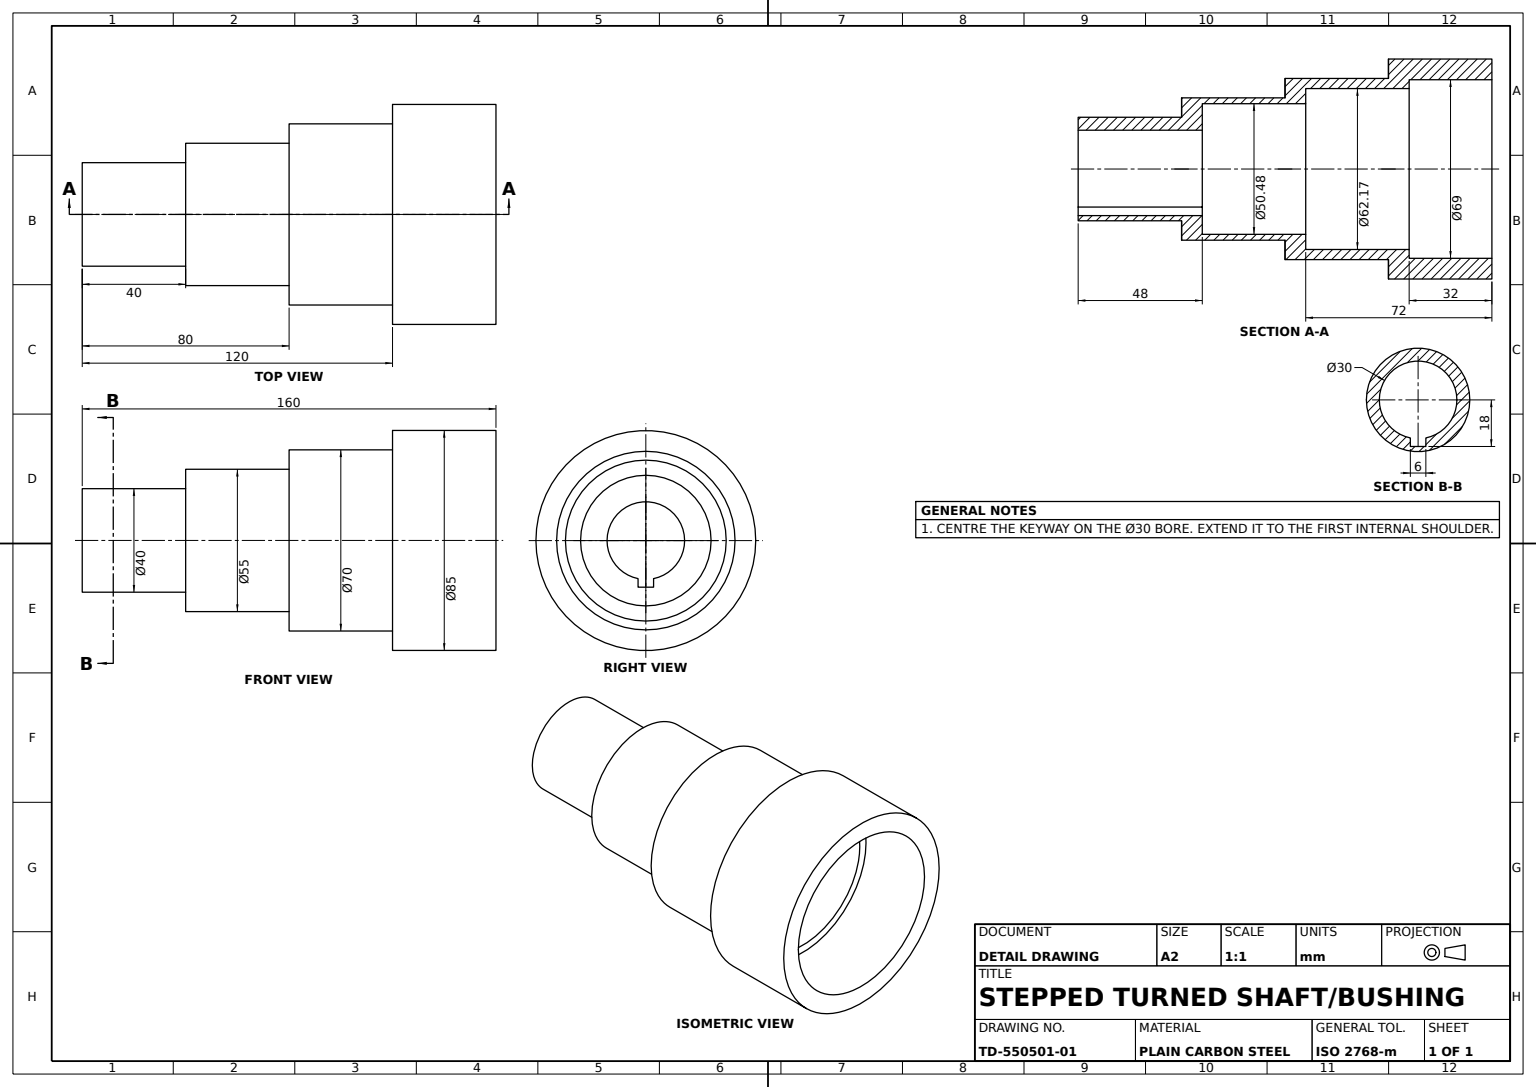
SolidWorks part; units mm, degrees
material "Plain Carbon Steel"
ref_plane "Front Plane" through (0, 0, 0) normal (0, 0, 1) x (1, 0, 0)
ref_plane "Top Plane" through (0, 0, 0) normal (0, 1, 0) x (1, 0, 0)
ref_plane "Right Plane" through (0, 0, 0) normal (1, 0, 0) x (0, 0, -1)
sketch "Stepped Profile Sketch" plane through (0, 0, 0) normal (0, 1, 0) x (1, 0, 0)
  line L1 (-80, 15.0355) -> (-80, 35.0355)
  line L2 (-80, 35.0355) -> (-40, 35.0355)
  line L3 (-40, 35.0355) -> (-40, 42.5355)
  line L4 (-40, 42.5355) -> (0, 42.5355)
  line L5 (0, 42.5355) -> (0, 50.0355)
  line L6 (0, 50.0355) -> (40, 50.0355)
  line L7 (40, 50.0355) -> (40, 57.5355)
  line L8 (40, 57.5355) -> (80, 57.5355)
  line L9 (80, 57.5355) -> (80, 49.5355)
  line L10 (80, 49.5355) -> (48, 49.5355)
  line L11 (48, 49.5355) -> (48, 46.1228)
  line L12 (48, 46.1228) -> (8, 46.1228)
  line L13 (8, 46.1228) -> (8, 40.2736)
  line L14 (8, 40.2736) -> (-32, 40.2736)
  line L15 (-32, 40.2736) -> (-32, 24.0831)
  line L16 (-32, 24.0831) -> (40, 24.0831)
  line L17 (40, 24.0831) -> (40, 15.0355)
  line L18 (40, 15.0355) -> (-80, 15.0355)
  dimension "D1" = 20
  dimension "D2" = 40
  dimension "D3" = 40
  dimension "D4" = 40
  dimension "D5" = 40
  dimension "D6" = 120
  dimension "D7" = 8
  dimension "D8" = 8
  dimension "D9" = 8
  dimension "D10" = 8
  dimension "D11" = 9.0476
  dimension "D12" = 27.5
  dimension "D13" = 35
  dimension "D14" = 3.4127
  dimension "85/2" = 42.5
  dimension "D15" = 5.8492
  dimension "D16" = 15.0355
revolve "Stepped Pulley Body" add sketch "Stepped Profile Sketch" angle 360 about L18
sketch "End Bore Sketch" plane through (-80, 0, 0) normal (-1, 0, 0) x (0, 0, 1)
  line L1 (-15.0355, -18) -> (-12.0355, -18)
  line L2 (-15.0355, -18) -> (-18.0355, -18)
  line L3 (-12.0355, -14.6969) -> (-12.0355, -18)
  line L4 (-18.0355, -14.6969) -> (-18.0355, -18)
  arc A0 (-12.0355, -14.6969) -> (-18.0355, -14.6969) centre (-15.0355, 0) ccw
  circle A1 centre (-15.0355, 0) radius 20 construction
  dimension "D1" = 30
  dimension "D2" = 3
  dimension "D3" = 18
extrude "End Bore 30 Deep" cut sketch "End Bore Sketch" against normal through all
